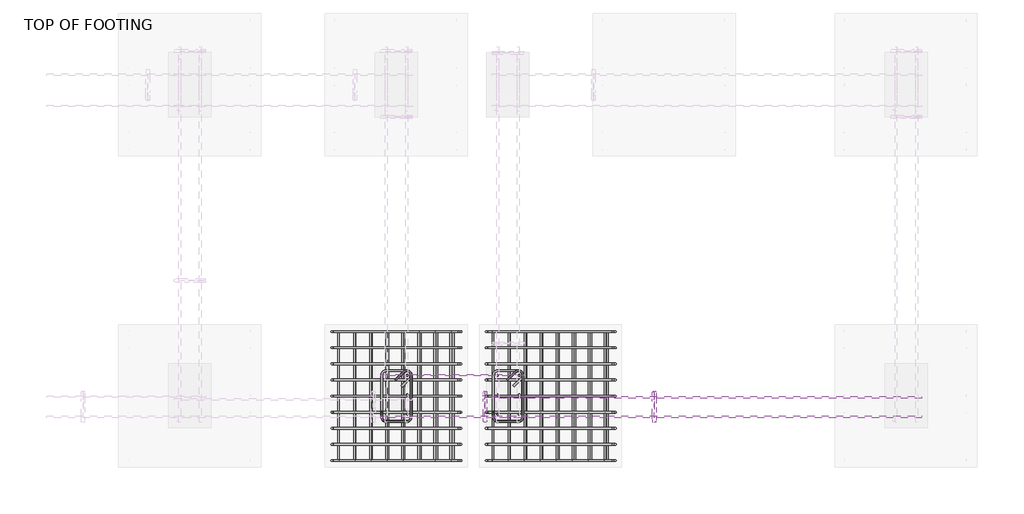
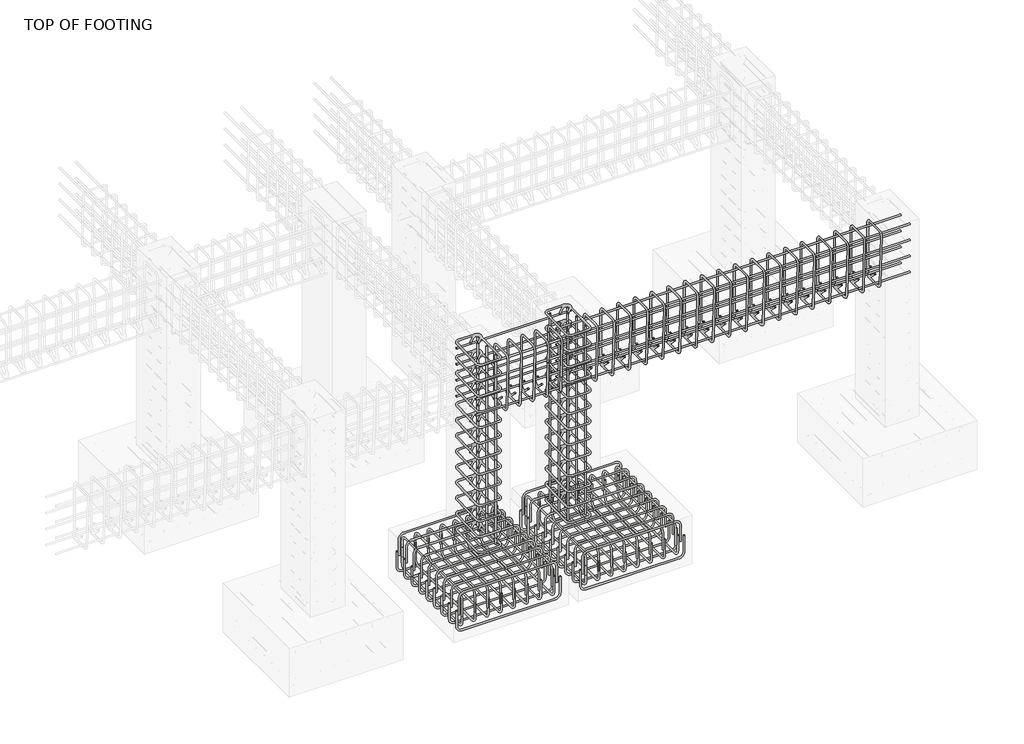
# One storey, part 3 of 19: 19 reinforcing bars.
"""IFC4 building model written with IfcOpenShell, lengths in millimetres."""

from ifc_helpers import new_model, si_unit, point, frame, origin, place, context, project, spatial, polyline, circle_curve, trimmed, segment, composite_curve, source, transform, mapped, element, save
from ifc_brep_helpers import swept_disk

model = new_model("IFC4")

# Units and contexts
model_context = context("Model", 3, world=origin())
ifc_project = project(units=[si_unit("LENGTHUNIT", "METRE", prefix="MILLI")], contexts=[model_context])

# Site, building, storey
site = spatial("IfcSite", under=ifc_project)
building = spatial("IfcBuilding", under=site)
storey = spatial("IfcBuildingStorey", under=building, Name="TOP OF FOOTING", Elevation=-1828.8)

# Reinforcing bars
placement = place(None, origin())
reinforcing_bar_shape = source(origin(), model_context, "Body", "SolidModel", [
    swept_disk(composite_curve([segment(polyline([(-418.7814918, -464.2751006, -2026.8103972), (-418.7814918, -464.2751006, -2174.1103972)]), True, "CONTINUOUS"), segment(trimmed(circle_curve(frame((-465.1314918, -464.2751006, -2174.1103972), z_axis=(0.0, 1.0, 0.0), x_axis=(46.349999999999966, 0.0, 0.0)), 46.35), [point((-418.7814918, -464.2751006, -2174.1103972))], [point((-465.1314918, -464.2751006, -2220.4603972))], True, "CARTESIAN"), True, "CONTINUOUS"), segment(polyline([(-465.1314918, -464.2751006, -2220.4603972), (-1279.7314918, -464.2751006, -2220.4603972)]), True, "CONTINUOUS"), segment(trimmed(circle_curve(frame((-1279.7314918, -464.2751006, -2174.1103972), z_axis=(0.0, 1.0, 0.0), x_axis=(0.0, 0.0, -46.34999999999991)), 46.35), [point((-1279.7314918, -464.2751006, -2220.4603972))], [point((-1326.0814918, -464.2751006, -2174.1103972))], True, "CARTESIAN"), True, "CONTINUOUS"), segment(polyline([(-1326.0814918, -464.2751006, -2174.1103972), (-1326.0814918, -464.2751006, -2026.8103972)]), True, "CONTINUOUS")], self_intersect=False), 6.35),
])
element("IfcReinforcingBar", 1, at=placement, inside=storey, context=model_context, shape_type="MappedRepresentation", body=[
    mapped(reinforcing_bar_shape, transform((0.0, 0.0, 0.0), x_axis=(1.0, 0.0, 0.0), y_axis=(0.0, 1.0, 0.0), z_axis=(0.0, 0.0, 1.0))),
    mapped(reinforcing_bar_shape, transform((0.0, -113.4125, 0.0), x_axis=(1.0, 0.0, 0.0), y_axis=(0.0, 1.0, 0.0), z_axis=(0.0, 0.0, 1.0))),
    mapped(reinforcing_bar_shape, transform((0.0, -226.825, 0.0), x_axis=(1.0, 0.0, 0.0), y_axis=(0.0, 1.0, 0.0), z_axis=(0.0, 0.0, 1.0))),
    mapped(reinforcing_bar_shape, transform((0.0, -340.2375, 0.0), x_axis=(1.0, 0.0, 0.0), y_axis=(0.0, 1.0, 0.0), z_axis=(0.0, 0.0, 1.0))),
    mapped(reinforcing_bar_shape, transform((0.0, -453.65, 0.0), x_axis=(1.0, 0.0, 0.0), y_axis=(0.0, 1.0, 0.0), z_axis=(0.0, 0.0, 1.0))),
    mapped(reinforcing_bar_shape, transform((0.0, -567.0625, 0.0), x_axis=(1.0, 0.0, 0.0), y_axis=(0.0, 1.0, 0.0), z_axis=(0.0, 0.0, 1.0))),
    mapped(reinforcing_bar_shape, transform((0.0, -680.475, 0.0), x_axis=(1.0, 0.0, 0.0), y_axis=(0.0, 1.0, 0.0), z_axis=(0.0, 0.0, 1.0))),
    mapped(reinforcing_bar_shape, transform((0.0, -793.8875, 0.0), x_axis=(1.0, 0.0, 0.0), y_axis=(0.0, 1.0, 0.0), z_axis=(0.0, 0.0, 1.0))),
    mapped(reinforcing_bar_shape, transform((0.0, -907.3, 0.0), x_axis=(1.0, 0.0, 0.0), y_axis=(0.0, 1.0, 0.0), z_axis=(0.0, 0.0, 1.0))),
])
reinforcing_bar_2_shape = source(origin(), model_context, "Body", "SolidModel", [
    swept_disk(composite_curve([segment(polyline([(-1306.5435207, -464.2751006, -2068.8), (-1306.5435207, -464.2751006, -1921.5)]), True, "CONTINUOUS"), segment(trimmed(circle_curve(frame((-1260.1935207, -464.2751006, -1921.5), z_axis=(0.0, 1.0, 0.0), x_axis=(-46.350000000000136, 0.0, 0.0)), 46.35), [point((-1306.5435207, -464.2751006, -1921.5))], [point((-1260.1935207, -464.2751006, -1875.15))], True, "CARTESIAN"), True, "CONTINUOUS"), segment(polyline([(-1260.1935207, -464.2751006, -1875.15), (-495.0610019, -464.2751006, -1875.15)]), True, "CONTINUOUS"), segment(trimmed(circle_curve(frame((-495.0610019, -464.2751006, -1921.5), z_axis=(0.0, 1.0, 0.0), x_axis=(0.0, 0.0, 46.34999999999991)), 46.35), [point((-495.0610019, -464.2751006, -1875.15))], [point((-448.7110019, -464.2751006, -1921.5))], True, "CARTESIAN"), True, "CONTINUOUS"), segment(polyline([(-448.7110019, -464.2751006, -1921.5), (-448.7110019, -464.2751006, -2068.8)]), True, "CONTINUOUS")], self_intersect=False), 6.35),
])
element("IfcReinforcingBar", 2, at=placement, inside=storey, context=model_context, shape_type="MappedRepresentation", body=[
    mapped(reinforcing_bar_2_shape, transform((0.0, 0.0, 0.0), x_axis=(1.0, 0.0, 0.0), y_axis=(0.0, 1.0, 0.0), z_axis=(0.0, 0.0, 1.0))),
    mapped(reinforcing_bar_2_shape, transform((0.0, -113.4125, 0.0), x_axis=(1.0, 0.0, 0.0), y_axis=(0.0, 1.0, 0.0), z_axis=(0.0, 0.0, 1.0))),
    mapped(reinforcing_bar_2_shape, transform((0.0, -226.825, 0.0), x_axis=(1.0, 0.0, 0.0), y_axis=(0.0, 1.0, 0.0), z_axis=(0.0, 0.0, 1.0))),
    mapped(reinforcing_bar_2_shape, transform((0.0, -340.2375, 0.0), x_axis=(1.0, 0.0, 0.0), y_axis=(0.0, 1.0, 0.0), z_axis=(0.0, 0.0, 1.0))),
    mapped(reinforcing_bar_2_shape, transform((0.0, -453.65, 0.0), x_axis=(1.0, 0.0, 0.0), y_axis=(0.0, 1.0, 0.0), z_axis=(0.0, 0.0, 1.0))),
    mapped(reinforcing_bar_2_shape, transform((0.0, -567.0625, 0.0), x_axis=(1.0, 0.0, 0.0), y_axis=(0.0, 1.0, 0.0), z_axis=(0.0, 0.0, 1.0))),
    mapped(reinforcing_bar_2_shape, transform((0.0, -680.475, 0.0), x_axis=(1.0, 0.0, 0.0), y_axis=(0.0, 1.0, 0.0), z_axis=(0.0, 0.0, 1.0))),
    mapped(reinforcing_bar_2_shape, transform((0.0, -793.8875, 0.0), x_axis=(1.0, 0.0, 0.0), y_axis=(0.0, 1.0, 0.0), z_axis=(0.0, 0.0, 1.0))),
    mapped(reinforcing_bar_2_shape, transform((0.0, -907.3, 0.0), x_axis=(1.0, 0.0, 0.0), y_axis=(0.0, 1.0, 0.0), z_axis=(0.0, 0.0, 1.0))),
])
reinforcing_bar_3_shape = source(origin(), model_context, "Body", "SolidModel", [
    swept_disk(composite_curve([segment(polyline([(-491.2862984, -464.2751006, -2090.0818702), (-491.2862984, -464.2751006, -1942.7818702)]), True, "CONTINUOUS"), segment(trimmed(circle_curve(frame((-491.2862984, -510.6251006, -1942.7818702), z_axis=(1.0, 0.0, 0.0), x_axis=(0.0, 46.35000000000002, 0.0)), 46.35), [point((-491.2862984, -464.2751006, -1942.7818702))], [point((-491.2862984, -510.6251006, -1896.4318702))], True, "CARTESIAN"), True, "CONTINUOUS"), segment(polyline([(-491.2862984, -510.6251006, -1896.4318702), (-491.2862984, -1325.2251006, -1896.4318702)]), True, "CONTINUOUS"), segment(trimmed(circle_curve(frame((-491.2862984, -1325.2251006, -1942.7818702), z_axis=(1.0, 0.0, 0.0), x_axis=(0.0, 0.0, 46.34999999999991)), 46.35), [point((-491.2862984, -1325.2251006, -1896.4318702))], [point((-491.2862984, -1371.5751006, -1942.7818702))], True, "CARTESIAN"), True, "CONTINUOUS"), segment(polyline([(-491.2862984, -1371.5751006, -1942.7818702), (-491.2862984, -1371.5751006, -2090.0818702)]), True, "CONTINUOUS")], self_intersect=False), 6.35),
])
element("IfcReinforcingBar", 3, at=placement, inside=storey, context=model_context, shape_type="MappedRepresentation", body=[
    mapped(reinforcing_bar_3_shape, transform((0.0, 0.0, 0.0), x_axis=(1.0, 0.0, 0.0), y_axis=(0.0, 1.0, 0.0), z_axis=(0.0, 0.0, 1.0))),
    mapped(reinforcing_bar_3_shape, transform((-112.5756498, 0.0, 0.0), x_axis=(1.0, 0.0, 0.0), y_axis=(0.0, 1.0, 0.0), z_axis=(0.0, 0.0, 1.0))),
    mapped(reinforcing_bar_3_shape, transform((-225.1512997, 0.0, 0.0), x_axis=(1.0, 0.0, 0.0), y_axis=(0.0, 1.0, 0.0), z_axis=(0.0, 0.0, 1.0))),
    mapped(reinforcing_bar_3_shape, transform((-337.7269495, 0.0, 0.0), x_axis=(1.0, 0.0, 0.0), y_axis=(0.0, 1.0, 0.0), z_axis=(0.0, 0.0, 1.0))),
    mapped(reinforcing_bar_3_shape, transform((-450.3025994, 0.0, 0.0), x_axis=(1.0, 0.0, 0.0), y_axis=(0.0, 1.0, 0.0), z_axis=(0.0, 0.0, 1.0))),
    mapped(reinforcing_bar_3_shape, transform((-562.8782492, 0.0, 0.0), x_axis=(1.0, 0.0, 0.0), y_axis=(0.0, 1.0, 0.0), z_axis=(0.0, 0.0, 1.0))),
    mapped(reinforcing_bar_3_shape, transform((-675.4538991, 0.0, 0.0), x_axis=(1.0, 0.0, 0.0), y_axis=(0.0, 1.0, 0.0), z_axis=(0.0, 0.0, 1.0))),
    mapped(reinforcing_bar_3_shape, transform((-788.0295489, 0.0, 0.0), x_axis=(1.0, 0.0, 0.0), y_axis=(0.0, 1.0, 0.0), z_axis=(0.0, 0.0, 1.0))),
])
reinforcing_bar_4_shape = source(origin(), model_context, "Body", "SolidModel", [
    swept_disk(composite_curve([segment(polyline([(-1279.3158473, -464.2751006, -2000.9061905), (-1279.3158473, -464.2751006, -2148.2061905)]), True, "CONTINUOUS"), segment(trimmed(circle_curve(frame((-1279.3158473, -510.6251006, -2148.2061905), z_axis=(-1.0, 0.0, 0.0), x_axis=(0.0, 46.35000000000002, 0.0)), 46.35), [point((-1279.3158473, -464.2751006, -2148.2061905))], [point((-1279.3158473, -510.6251006, -2194.5561905))], True, "CARTESIAN"), True, "CONTINUOUS"), segment(polyline([(-1279.3158473, -510.6251006, -2194.5561905), (-1279.3158473, -1325.2251006, -2194.5561905)]), True, "CONTINUOUS"), segment(trimmed(circle_curve(frame((-1279.3158473, -1325.2251006, -2148.2061905), z_axis=(-1.0, 0.0, 0.0), x_axis=(0.0, 0.0, -46.34999999999991)), 46.35), [point((-1279.3158473, -1325.2251006, -2194.5561905))], [point((-1279.3158473, -1371.5751006, -2148.2061905))], True, "CARTESIAN"), True, "CONTINUOUS"), segment(polyline([(-1279.3158473, -1371.5751006, -2148.2061905), (-1279.3158473, -1371.5751006, -2000.9061905)]), True, "CONTINUOUS")], self_intersect=False), 6.35),
])
element("IfcReinforcingBar", 4, at=placement, inside=storey, context=model_context, shape_type="MappedRepresentation", body=[
    mapped(reinforcing_bar_4_shape, transform((0.0, 0.0, 0.0), x_axis=(1.0, 0.0, 0.0), y_axis=(0.0, 1.0, 0.0), z_axis=(0.0, 0.0, 1.0))),
    mapped(reinforcing_bar_4_shape, transform((115.0727115, 0.0, 0.0), x_axis=(1.0, 0.0, 0.0), y_axis=(0.0, 1.0, 0.0), z_axis=(0.0, 0.0, 1.0))),
    mapped(reinforcing_bar_4_shape, transform((230.145423, 0.0, 0.0), x_axis=(1.0, 0.0, 0.0), y_axis=(0.0, 1.0, 0.0), z_axis=(0.0, 0.0, 1.0))),
    mapped(reinforcing_bar_4_shape, transform((345.2181344, 0.0, 0.0), x_axis=(1.0, 0.0, 0.0), y_axis=(0.0, 1.0, 0.0), z_axis=(0.0, 0.0, 1.0))),
    mapped(reinforcing_bar_4_shape, transform((460.2908459, 0.0, 0.0), x_axis=(1.0, 0.0, 0.0), y_axis=(0.0, 1.0, 0.0), z_axis=(0.0, 0.0, 1.0))),
    mapped(reinforcing_bar_4_shape, transform((575.3635574, 0.0, 0.0), x_axis=(1.0, 0.0, 0.0), y_axis=(0.0, 1.0, 0.0), z_axis=(0.0, 0.0, 1.0))),
    mapped(reinforcing_bar_4_shape, transform((690.4362689, 0.0, 0.0), x_axis=(1.0, 0.0, 0.0), y_axis=(0.0, 1.0, 0.0), z_axis=(0.0, 0.0, 1.0))),
    mapped(reinforcing_bar_4_shape, transform((805.5089804, 0.0, 0.0), x_axis=(1.0, 0.0, 0.0), y_axis=(0.0, 1.0, 0.0), z_axis=(0.0, 0.0, 1.0))),
])
reinforcing_bar_5_shape = source(origin(), model_context, "Body", "SolidModel", [
    swept_disk(composite_curve([segment(polyline([(-1504.0266954, -464.2751006, -2026.8103972), (-1504.0266954, -464.2751006, -2174.1103972)]), True, "CONTINUOUS"), segment(trimmed(circle_curve(frame((-1550.3766954, -464.2751006, -2174.1103972), z_axis=(0.0, 1.0, 0.0), x_axis=(46.34999999999991, 0.0, 0.0)), 46.35), [point((-1504.0266954, -464.2751006, -2174.1103972))], [point((-1550.3766954, -464.2751006, -2220.4603972))], True, "CARTESIAN"), True, "CONTINUOUS"), segment(polyline([(-1550.3766954, -464.2751006, -2220.4603972), (-2364.9766954, -464.2751006, -2220.4603972)]), True, "CONTINUOUS"), segment(trimmed(circle_curve(frame((-2364.9766954, -464.2751006, -2174.1103972), z_axis=(0.0, 1.0, 0.0), x_axis=(0.0, 0.0, -46.34999999999991)), 46.35), [point((-2364.9766954, -464.2751006, -2220.4603972))], [point((-2411.3266954, -464.2751006, -2174.1103972))], True, "CARTESIAN"), True, "CONTINUOUS"), segment(polyline([(-2411.3266954, -464.2751006, -2174.1103972), (-2411.3266954, -464.2751006, -2026.8103972)]), True, "CONTINUOUS")], self_intersect=False), 6.35),
])
element("IfcReinforcingBar", 5, at=placement, inside=storey, context=model_context, shape_type="MappedRepresentation", body=[
    mapped(reinforcing_bar_5_shape, transform((0.0, 0.0, 0.0), x_axis=(1.0, 0.0, 0.0), y_axis=(0.0, 1.0, 0.0), z_axis=(0.0, 0.0, 1.0))),
    mapped(reinforcing_bar_5_shape, transform((0.0, -113.4125, 0.0), x_axis=(1.0, 0.0, 0.0), y_axis=(0.0, 1.0, 0.0), z_axis=(0.0, 0.0, 1.0))),
    mapped(reinforcing_bar_5_shape, transform((0.0, -226.825, 0.0), x_axis=(1.0, 0.0, 0.0), y_axis=(0.0, 1.0, 0.0), z_axis=(0.0, 0.0, 1.0))),
    mapped(reinforcing_bar_5_shape, transform((0.0, -340.2375, 0.0), x_axis=(1.0, 0.0, 0.0), y_axis=(0.0, 1.0, 0.0), z_axis=(0.0, 0.0, 1.0))),
    mapped(reinforcing_bar_5_shape, transform((0.0, -453.65, 0.0), x_axis=(1.0, 0.0, 0.0), y_axis=(0.0, 1.0, 0.0), z_axis=(0.0, 0.0, 1.0))),
    mapped(reinforcing_bar_5_shape, transform((0.0, -567.0625, 0.0), x_axis=(1.0, 0.0, 0.0), y_axis=(0.0, 1.0, 0.0), z_axis=(0.0, 0.0, 1.0))),
    mapped(reinforcing_bar_5_shape, transform((0.0, -680.475, 0.0), x_axis=(1.0, 0.0, 0.0), y_axis=(0.0, 1.0, 0.0), z_axis=(0.0, 0.0, 1.0))),
    mapped(reinforcing_bar_5_shape, transform((0.0, -793.8875, 0.0), x_axis=(1.0, 0.0, 0.0), y_axis=(0.0, 1.0, 0.0), z_axis=(0.0, 0.0, 1.0))),
    mapped(reinforcing_bar_5_shape, transform((0.0, -907.3, 0.0), x_axis=(1.0, 0.0, 0.0), y_axis=(0.0, 1.0, 0.0), z_axis=(0.0, 0.0, 1.0))),
])
reinforcing_bar_6_shape = source(origin(), model_context, "Body", "SolidModel", [
    swept_disk(composite_curve([segment(polyline([(-2391.7887242, -464.2751006, -2068.8), (-2391.7887242, -464.2751006, -1921.5)]), True, "CONTINUOUS"), segment(trimmed(circle_curve(frame((-2345.4387242, -464.2751006, -1921.5), z_axis=(0.0, 1.0, 0.0), x_axis=(-46.350000000000364, 0.0, 0.0)), 46.35), [point((-2391.7887242, -464.2751006, -1921.5))], [point((-2345.4387242, -464.2751006, -1875.15))], True, "CARTESIAN"), True, "CONTINUOUS"), segment(polyline([(-2345.4387242, -464.2751006, -1875.15), (-1580.3062054, -464.2751006, -1875.15)]), True, "CONTINUOUS"), segment(trimmed(circle_curve(frame((-1580.3062054, -464.2751006, -1921.5), z_axis=(0.0, 1.0, 0.0), x_axis=(0.0, 0.0, 46.34999999999991)), 46.35), [point((-1580.3062054, -464.2751006, -1875.15))], [point((-1533.9562054, -464.2751006, -1921.5))], True, "CARTESIAN"), True, "CONTINUOUS"), segment(polyline([(-1533.9562054, -464.2751006, -1921.5), (-1533.9562054, -464.2751006, -2068.8)]), True, "CONTINUOUS")], self_intersect=False), 6.35),
])
element("IfcReinforcingBar", 6, at=placement, inside=storey, context=model_context, shape_type="MappedRepresentation", body=[
    mapped(reinforcing_bar_6_shape, transform((0.0, 0.0, 0.0), x_axis=(1.0, 0.0, 0.0), y_axis=(0.0, 1.0, 0.0), z_axis=(0.0, 0.0, 1.0))),
    mapped(reinforcing_bar_6_shape, transform((0.0, -113.4125, 0.0), x_axis=(1.0, 0.0, 0.0), y_axis=(0.0, 1.0, 0.0), z_axis=(0.0, 0.0, 1.0))),
    mapped(reinforcing_bar_6_shape, transform((0.0, -226.825, 0.0), x_axis=(1.0, 0.0, 0.0), y_axis=(0.0, 1.0, 0.0), z_axis=(0.0, 0.0, 1.0))),
    mapped(reinforcing_bar_6_shape, transform((0.0, -340.2375, 0.0), x_axis=(1.0, 0.0, 0.0), y_axis=(0.0, 1.0, 0.0), z_axis=(0.0, 0.0, 1.0))),
    mapped(reinforcing_bar_6_shape, transform((0.0, -453.65, 0.0), x_axis=(1.0, 0.0, 0.0), y_axis=(0.0, 1.0, 0.0), z_axis=(0.0, 0.0, 1.0))),
    mapped(reinforcing_bar_6_shape, transform((0.0, -567.0625, 0.0), x_axis=(1.0, 0.0, 0.0), y_axis=(0.0, 1.0, 0.0), z_axis=(0.0, 0.0, 1.0))),
    mapped(reinforcing_bar_6_shape, transform((0.0, -680.475, 0.0), x_axis=(1.0, 0.0, 0.0), y_axis=(0.0, 1.0, 0.0), z_axis=(0.0, 0.0, 1.0))),
    mapped(reinforcing_bar_6_shape, transform((0.0, -793.8875, 0.0), x_axis=(1.0, 0.0, 0.0), y_axis=(0.0, 1.0, 0.0), z_axis=(0.0, 0.0, 1.0))),
    mapped(reinforcing_bar_6_shape, transform((0.0, -907.3, 0.0), x_axis=(1.0, 0.0, 0.0), y_axis=(0.0, 1.0, 0.0), z_axis=(0.0, 0.0, 1.0))),
])
reinforcing_bar_7_shape = source(origin(), model_context, "Body", "SolidModel", [
    swept_disk(composite_curve([segment(polyline([(-1576.531502, -464.2751006, -2090.0818702), (-1576.531502, -464.2751006, -1942.7818702)]), True, "CONTINUOUS"), segment(trimmed(circle_curve(frame((-1576.531502, -510.6251006, -1942.7818702), z_axis=(1.0, 0.0, 0.0), x_axis=(0.0, 46.35000000000002, 0.0)), 46.35), [point((-1576.531502, -464.2751006, -1942.7818702))], [point((-1576.531502, -510.6251006, -1896.4318702))], True, "CARTESIAN"), True, "CONTINUOUS"), segment(polyline([(-1576.531502, -510.6251006, -1896.4318702), (-1576.531502, -1325.2251006, -1896.4318702)]), True, "CONTINUOUS"), segment(trimmed(circle_curve(frame((-1576.531502, -1325.2251006, -1942.7818702), z_axis=(1.0, 0.0, 0.0), x_axis=(0.0, 0.0, 46.34999999999991)), 46.35), [point((-1576.531502, -1325.2251006, -1896.4318702))], [point((-1576.531502, -1371.5751006, -1942.7818702))], True, "CARTESIAN"), True, "CONTINUOUS"), segment(polyline([(-1576.531502, -1371.5751006, -1942.7818702), (-1576.531502, -1371.5751006, -2090.0818702)]), True, "CONTINUOUS")], self_intersect=False), 6.35),
])
element("IfcReinforcingBar", 7, at=placement, inside=storey, context=model_context, shape_type="MappedRepresentation", body=[
    mapped(reinforcing_bar_7_shape, transform((0.0, 0.0, 0.0), x_axis=(1.0, 0.0, 0.0), y_axis=(0.0, 1.0, 0.0), z_axis=(0.0, 0.0, 1.0))),
    mapped(reinforcing_bar_7_shape, transform((-112.5756498, 0.0, 0.0), x_axis=(1.0, 0.0, 0.0), y_axis=(0.0, 1.0, 0.0), z_axis=(0.0, 0.0, 1.0))),
    mapped(reinforcing_bar_7_shape, transform((-225.1512997, 0.0, 0.0), x_axis=(1.0, 0.0, 0.0), y_axis=(0.0, 1.0, 0.0), z_axis=(0.0, 0.0, 1.0))),
    mapped(reinforcing_bar_7_shape, transform((-337.7269495, 0.0, 0.0), x_axis=(1.0, 0.0, 0.0), y_axis=(0.0, 1.0, 0.0), z_axis=(0.0, 0.0, 1.0))),
    mapped(reinforcing_bar_7_shape, transform((-450.3025994, 0.0, 0.0), x_axis=(1.0, 0.0, 0.0), y_axis=(0.0, 1.0, 0.0), z_axis=(0.0, 0.0, 1.0))),
    mapped(reinforcing_bar_7_shape, transform((-562.8782492, 0.0, 0.0), x_axis=(1.0, 0.0, 0.0), y_axis=(0.0, 1.0, 0.0), z_axis=(0.0, 0.0, 1.0))),
    mapped(reinforcing_bar_7_shape, transform((-675.4538991, 0.0, 0.0), x_axis=(1.0, 0.0, 0.0), y_axis=(0.0, 1.0, 0.0), z_axis=(0.0, 0.0, 1.0))),
    mapped(reinforcing_bar_7_shape, transform((-788.0295489, 0.0, 0.0), x_axis=(1.0, 0.0, 0.0), y_axis=(0.0, 1.0, 0.0), z_axis=(0.0, 0.0, 1.0))),
])
reinforcing_bar_8_shape = source(origin(), model_context, "Body", "SolidModel", [
    swept_disk(composite_curve([segment(polyline([(-2364.5610509, -464.2751006, -2000.9061905), (-2364.5610509, -464.2751006, -2148.2061905)]), True, "CONTINUOUS"), segment(trimmed(circle_curve(frame((-2364.5610509, -510.6251006, -2148.2061905), z_axis=(-1.0, 0.0, 0.0), x_axis=(0.0, 46.35000000000002, 0.0)), 46.35), [point((-2364.5610509, -464.2751006, -2148.2061905))], [point((-2364.5610509, -510.6251006, -2194.5561905))], True, "CARTESIAN"), True, "CONTINUOUS"), segment(polyline([(-2364.5610509, -510.6251006, -2194.5561905), (-2364.5610509, -1325.2251006, -2194.5561905)]), True, "CONTINUOUS"), segment(trimmed(circle_curve(frame((-2364.5610509, -1325.2251006, -2148.2061905), z_axis=(-1.0, 0.0, 0.0), x_axis=(0.0, 0.0, -46.34999999999991)), 46.35), [point((-2364.5610509, -1325.2251006, -2194.5561905))], [point((-2364.5610509, -1371.5751006, -2148.2061905))], True, "CARTESIAN"), True, "CONTINUOUS"), segment(polyline([(-2364.5610509, -1371.5751006, -2148.2061905), (-2364.5610509, -1371.5751006, -2000.9061905)]), True, "CONTINUOUS")], self_intersect=False), 6.35),
])
element("IfcReinforcingBar", 8, at=placement, inside=storey, context=model_context, shape_type="MappedRepresentation", body=[
    mapped(reinforcing_bar_8_shape, transform((0.0, 0.0, 0.0), x_axis=(1.0, 0.0, 0.0), y_axis=(0.0, 1.0, 0.0), z_axis=(0.0, 0.0, 1.0))),
    mapped(reinforcing_bar_8_shape, transform((115.0727115, 0.0, 0.0), x_axis=(1.0, 0.0, 0.0), y_axis=(0.0, 1.0, 0.0), z_axis=(0.0, 0.0, 1.0))),
    mapped(reinforcing_bar_8_shape, transform((230.145423, 0.0, 0.0), x_axis=(1.0, 0.0, 0.0), y_axis=(0.0, 1.0, 0.0), z_axis=(0.0, 0.0, 1.0))),
    mapped(reinforcing_bar_8_shape, transform((345.2181344, 0.0, 0.0), x_axis=(1.0, 0.0, 0.0), y_axis=(0.0, 1.0, 0.0), z_axis=(0.0, 0.0, 1.0))),
    mapped(reinforcing_bar_8_shape, transform((460.2908459, 0.0, 0.0), x_axis=(1.0, 0.0, 0.0), y_axis=(0.0, 1.0, 0.0), z_axis=(0.0, 0.0, 1.0))),
    mapped(reinforcing_bar_8_shape, transform((575.3635574, 0.0, 0.0), x_axis=(1.0, 0.0, 0.0), y_axis=(0.0, 1.0, 0.0), z_axis=(0.0, 0.0, 1.0))),
    mapped(reinforcing_bar_8_shape, transform((690.4362689, 0.0, 0.0), x_axis=(1.0, 0.0, 0.0), y_axis=(0.0, 1.0, 0.0), z_axis=(0.0, 0.0, 1.0))),
    mapped(reinforcing_bar_8_shape, transform((805.5089804, 0.0, 0.0), x_axis=(1.0, 0.0, 0.0), y_axis=(0.0, 1.0, 0.0), z_axis=(0.0, 0.0, 1.0))),
])
reinforcing_bar_9_shape = source(origin(), model_context, "Body", "SolidModel", [
    swept_disk(composite_curve([segment(polyline([(-1963.2880559, -804.200866, -46.35), (-1907.544493, -748.457303, -46.35)]), True, "CONTINUOUS"), segment(trimmed(circle_curve(frame((-1885.3766954, -770.6251006, -46.35), z_axis=(0.0, 0.0, -1.0), x_axis=(-22.167797600000085, 22.16779759999997, 0.0)), 31.35), [point((-1907.544493, -748.457303, -46.35))], [point((-1854.0266954, -770.6251006, -46.35))], True, "CARTESIAN"), True, "CONTINUOUS"), segment(polyline([(-1854.0266954, -770.6251006, -46.35), (-1854.0266954, -1065.2251006, -46.35)]), True, "CONTINUOUS"), segment(trimmed(circle_curve(frame((-1885.3766954, -1065.2251006, -46.35), z_axis=(0.0, 0.0, -1.0), x_axis=(31.34999999999991, 0.0, 0.0)), 31.35), [point((-1854.0266954, -1065.2251006, -46.35))], [point((-1885.3766954, -1096.5751006, -46.35))], True, "CARTESIAN"), True, "CONTINUOUS"), segment(polyline([(-1885.3766954, -1096.5751006, -46.35), (-2029.9766954, -1096.5751006, -46.35)]), True, "CONTINUOUS"), segment(trimmed(circle_curve(frame((-2029.9766954, -1065.2448857, -45.2363875), z_axis=(0.0, 0.035521928334481916, -0.9993688971583016), x_axis=(0.0, -31.3302149000001, -1.1136125000000021)), 31.35), [point((-2029.9766954, -1096.5751006, -46.35))], [point((-2061.3266954, -1065.2448857, -45.2363875))], True, "CARTESIAN"), True, "CONTINUOUS"), segment(polyline([(-2061.3266954, -1065.2448857, -45.2363875), (-2061.3266954, -770.6053156, -34.7636125)]), True, "CONTINUOUS"), segment(trimmed(circle_curve(frame((-2029.9766954, -770.6053156, -34.7636125), z_axis=(0.0, 0.035521928334481916, -0.9993688971583016), x_axis=(-31.350000000000136, 0.0, 0.0)), 31.35), [point((-2061.3266954, -770.6053156, -34.7636125))], [point((-2029.9766954, -739.2751006, -33.65))], True, "CARTESIAN"), True, "CONTINUOUS"), segment(polyline([(-2029.9766954, -739.2751006, -33.65), (-1885.3766954, -739.2751006, -33.65)]), True, "CONTINUOUS"), segment(trimmed(circle_curve(frame((-1885.3766954, -770.6251006, -33.65), z_axis=(0.0, 0.0, -1.0), x_axis=(0.0, 31.350000000000023, 0.0)), 31.35), [point((-1885.3766954, -739.2751006, -33.65))], [point((-1863.2088978, -792.7928982, -33.65))], True, "CARTESIAN"), True, "CONTINUOUS"), segment(polyline([(-1863.2088978, -792.7928982, -33.65), (-1918.9524607, -848.5364612, -33.65)]), True, "CONTINUOUS")], self_intersect=False), 6.35),
])
element("IfcReinforcingBar", 9, at=placement, inside=storey, context=model_context, shape_type="MappedRepresentation", body=[
    mapped(reinforcing_bar_9_shape, transform((0.0, 0.0, 0.0), x_axis=(1.0, 0.0, 0.0), y_axis=(0.0, 1.0, 0.0), z_axis=(0.0, 0.0, 1.0))),
    mapped(reinforcing_bar_9_shape, transform((0.0, 0.0, -144.675), x_axis=(1.0, 0.0, 0.0), y_axis=(0.0, 1.0, 0.0), z_axis=(0.0, 0.0, 1.0))),
    mapped(reinforcing_bar_9_shape, transform((0.0, 0.0, -289.35), x_axis=(1.0, 0.0, 0.0), y_axis=(0.0, 1.0, 0.0), z_axis=(0.0, 0.0, 1.0))),
    mapped(reinforcing_bar_9_shape, transform((0.0, 0.0, -434.025), x_axis=(1.0, 0.0, 0.0), y_axis=(0.0, 1.0, 0.0), z_axis=(0.0, 0.0, 1.0))),
    mapped(reinforcing_bar_9_shape, transform((0.0, 0.0, -578.7), x_axis=(1.0, 0.0, 0.0), y_axis=(0.0, 1.0, 0.0), z_axis=(0.0, 0.0, 1.0))),
    mapped(reinforcing_bar_9_shape, transform((0.0, 0.0, -723.375), x_axis=(1.0, 0.0, 0.0), y_axis=(0.0, 1.0, 0.0), z_axis=(0.0, 0.0, 1.0))),
    mapped(reinforcing_bar_9_shape, transform((0.0, 0.0, -868.05), x_axis=(1.0, 0.0, 0.0), y_axis=(0.0, 1.0, 0.0), z_axis=(0.0, 0.0, 1.0))),
    mapped(reinforcing_bar_9_shape, transform((0.0, 0.0, -1012.725), x_axis=(1.0, 0.0, 0.0), y_axis=(0.0, 1.0, 0.0), z_axis=(0.0, 0.0, 1.0))),
    mapped(reinforcing_bar_9_shape, transform((0.0, 0.0, -1157.4), x_axis=(1.0, 0.0, 0.0), y_axis=(0.0, 1.0, 0.0), z_axis=(0.0, 0.0, 1.0))),
    mapped(reinforcing_bar_9_shape, transform((0.0, 0.0, -1302.075), x_axis=(1.0, 0.0, 0.0), y_axis=(0.0, 1.0, 0.0), z_axis=(0.0, 0.0, 1.0))),
    mapped(reinforcing_bar_9_shape, transform((0.0, 0.0, -1446.75), x_axis=(1.0, 0.0, 0.0), y_axis=(0.0, 1.0, 0.0), z_axis=(0.0, 0.0, 1.0))),
    mapped(reinforcing_bar_9_shape, transform((0.0, 0.0, -1591.425), x_axis=(1.0, 0.0, 0.0), y_axis=(0.0, 1.0, 0.0), z_axis=(0.0, 0.0, 1.0))),
    mapped(reinforcing_bar_9_shape, transform((0.0, 0.0, -1736.1), x_axis=(1.0, 0.0, 0.0), y_axis=(0.0, 1.0, 0.0), z_axis=(0.0, 0.0, 1.0))),
])
reinforcing_bar_10_shape = source(origin(), model_context, "Body", "SolidModel", [
    swept_disk(composite_curve([segment(polyline([(-1880.3766954, -772.4299352, -40.0), (-1880.3766954, -772.4299352, -1788.8)]), True, "CONTINUOUS")], self_intersect=False), 6.35),
])
element("IfcReinforcingBar", 10, at=placement, inside=storey, context=model_context, shape_type="MappedRepresentation", body=[
    mapped(reinforcing_bar_10_shape, transform((0.0, 0.0, 0.0), x_axis=(1.0, 0.0, 0.0), y_axis=(0.0, 1.0, 0.0), z_axis=(0.0, 0.0, 1.0))),
    mapped(reinforcing_bar_10_shape, transform((0.0, -136.8171118, 0.0), x_axis=(1.0, 0.0, 0.0), y_axis=(0.0, 1.0, 0.0), z_axis=(0.0, 0.0, 1.0))),
    mapped(reinforcing_bar_10_shape, transform((0.0, -273.6342236, 0.0), x_axis=(1.0, 0.0, 0.0), y_axis=(0.0, 1.0, 0.0), z_axis=(0.0, 0.0, 1.0))),
])
reinforcing_bar_11_shape = source(origin(), model_context, "Body", "SolidModel", [
    swept_disk(composite_curve([segment(polyline([(-1178.0428523, -804.200866, -46.35), (-1122.2992894, -748.457303, -46.35)]), True, "CONTINUOUS"), segment(trimmed(circle_curve(frame((-1100.1314918, -770.6251006, -46.35), z_axis=(0.0, 0.0, -1.0), x_axis=(-22.167797599999858, 22.16779759999997, 0.0)), 31.35), [point((-1122.2992894, -748.457303, -46.35))], [point((-1068.7814918, -770.6251006, -46.35))], True, "CARTESIAN"), True, "CONTINUOUS"), segment(polyline([(-1068.7814918, -770.6251006, -46.35), (-1068.7814918, -1065.2251006, -46.35)]), True, "CONTINUOUS"), segment(trimmed(circle_curve(frame((-1100.1314918, -1065.2251006, -46.35), z_axis=(0.0, 0.0, -1.0), x_axis=(31.350000000000136, 0.0, 0.0)), 31.35), [point((-1068.7814918, -1065.2251006, -46.35))], [point((-1100.1314918, -1096.5751006, -46.35))], True, "CARTESIAN"), True, "CONTINUOUS"), segment(polyline([(-1100.1314918, -1096.5751006, -46.35), (-1244.7314918, -1096.5751006, -46.35)]), True, "CONTINUOUS"), segment(trimmed(circle_curve(frame((-1244.7314918, -1065.2448857, -45.2363875), z_axis=(0.0, 0.035521928334481916, -0.9993688971583016), x_axis=(0.0, -31.3302149000001, -1.1136125000000021)), 31.35), [point((-1244.7314918, -1096.5751006, -46.35))], [point((-1276.0814918, -1065.2448857, -45.2363875))], True, "CARTESIAN"), True, "CONTINUOUS"), segment(polyline([(-1276.0814918, -1065.2448857, -45.2363875), (-1276.0814918, -770.6053156, -34.7636125)]), True, "CONTINUOUS"), segment(trimmed(circle_curve(frame((-1244.7314918, -770.6053156, -34.7636125), z_axis=(0.0, 0.035521928334481916, -0.9993688971583016), x_axis=(-31.350000000000136, 0.0, 0.0)), 31.35), [point((-1276.0814918, -770.6053156, -34.7636125))], [point((-1244.7314918, -739.2751006, -33.65))], True, "CARTESIAN"), True, "CONTINUOUS"), segment(polyline([(-1244.7314918, -739.2751006, -33.65), (-1100.1314918, -739.2751006, -33.65)]), True, "CONTINUOUS"), segment(trimmed(circle_curve(frame((-1100.1314918, -770.6251006, -33.65), z_axis=(0.0, 0.0, -1.0), x_axis=(0.0, 31.350000000000023, 0.0)), 31.35), [point((-1100.1314918, -739.2751006, -33.65))], [point((-1077.9636942, -792.7928982, -33.65))], True, "CARTESIAN"), True, "CONTINUOUS"), segment(polyline([(-1077.9636942, -792.7928982, -33.65), (-1133.7072572, -848.5364612, -33.65)]), True, "CONTINUOUS")], self_intersect=False), 6.35),
])
element("IfcReinforcingBar", 11, at=placement, inside=storey, context=model_context, shape_type="MappedRepresentation", body=[
    mapped(reinforcing_bar_11_shape, transform((0.0, 0.0, 0.0), x_axis=(1.0, 0.0, 0.0), y_axis=(0.0, 1.0, 0.0), z_axis=(0.0, 0.0, 1.0))),
    mapped(reinforcing_bar_11_shape, transform((0.0, 0.0, -144.675), x_axis=(1.0, 0.0, 0.0), y_axis=(0.0, 1.0, 0.0), z_axis=(0.0, 0.0, 1.0))),
    mapped(reinforcing_bar_11_shape, transform((0.0, 0.0, -289.35), x_axis=(1.0, 0.0, 0.0), y_axis=(0.0, 1.0, 0.0), z_axis=(0.0, 0.0, 1.0))),
    mapped(reinforcing_bar_11_shape, transform((0.0, 0.0, -434.025), x_axis=(1.0, 0.0, 0.0), y_axis=(0.0, 1.0, 0.0), z_axis=(0.0, 0.0, 1.0))),
    mapped(reinforcing_bar_11_shape, transform((0.0, 0.0, -578.7), x_axis=(1.0, 0.0, 0.0), y_axis=(0.0, 1.0, 0.0), z_axis=(0.0, 0.0, 1.0))),
    mapped(reinforcing_bar_11_shape, transform((0.0, 0.0, -723.375), x_axis=(1.0, 0.0, 0.0), y_axis=(0.0, 1.0, 0.0), z_axis=(0.0, 0.0, 1.0))),
    mapped(reinforcing_bar_11_shape, transform((0.0, 0.0, -868.05), x_axis=(1.0, 0.0, 0.0), y_axis=(0.0, 1.0, 0.0), z_axis=(0.0, 0.0, 1.0))),
    mapped(reinforcing_bar_11_shape, transform((0.0, 0.0, -1012.725), x_axis=(1.0, 0.0, 0.0), y_axis=(0.0, 1.0, 0.0), z_axis=(0.0, 0.0, 1.0))),
    mapped(reinforcing_bar_11_shape, transform((0.0, 0.0, -1157.4), x_axis=(1.0, 0.0, 0.0), y_axis=(0.0, 1.0, 0.0), z_axis=(0.0, 0.0, 1.0))),
    mapped(reinforcing_bar_11_shape, transform((0.0, 0.0, -1302.075), x_axis=(1.0, 0.0, 0.0), y_axis=(0.0, 1.0, 0.0), z_axis=(0.0, 0.0, 1.0))),
    mapped(reinforcing_bar_11_shape, transform((0.0, 0.0, -1446.75), x_axis=(1.0, 0.0, 0.0), y_axis=(0.0, 1.0, 0.0), z_axis=(0.0, 0.0, 1.0))),
    mapped(reinforcing_bar_11_shape, transform((0.0, 0.0, -1591.425), x_axis=(1.0, 0.0, 0.0), y_axis=(0.0, 1.0, 0.0), z_axis=(0.0, 0.0, 1.0))),
    mapped(reinforcing_bar_11_shape, transform((0.0, 0.0, -1736.1), x_axis=(1.0, 0.0, 0.0), y_axis=(0.0, 1.0, 0.0), z_axis=(0.0, 0.0, 1.0))),
])
reinforcing_bar_12_shape = source(origin(), model_context, "Body", "SolidModel", [
    swept_disk(composite_curve([segment(polyline([(-1095.1314918, -772.4299352, -40.0), (-1095.1314918, -772.4299352, -1788.8)]), True, "CONTINUOUS")], self_intersect=False), 6.35),
])
element("IfcReinforcingBar", 12, at=placement, inside=storey, context=model_context, shape_type="MappedRepresentation", body=[
    mapped(reinforcing_bar_12_shape, transform((0.0, 0.0, 0.0), x_axis=(1.0, 0.0, 0.0), y_axis=(0.0, 1.0, 0.0), z_axis=(0.0, 0.0, 1.0))),
    mapped(reinforcing_bar_12_shape, transform((0.0, -136.8171118, 0.0), x_axis=(1.0, 0.0, 0.0), y_axis=(0.0, 1.0, 0.0), z_axis=(0.0, 0.0, 1.0))),
    mapped(reinforcing_bar_12_shape, transform((0.0, -273.6342236, 0.0), x_axis=(1.0, 0.0, 0.0), y_axis=(0.0, 1.0, 0.0), z_axis=(0.0, 0.0, 1.0))),
])
reinforcing_bar_13_shape = source(origin(), model_context, "Body", "SolidModel", [
    swept_disk(composite_curve([segment(polyline([(-1247.2314918, -772.4299352, -40.0), (-1247.2314918, -772.4299352, -1788.8)]), True, "CONTINUOUS")], self_intersect=False), 6.35),
])
element("IfcReinforcingBar", 13, at=placement, inside=storey, context=model_context, shape_type="MappedRepresentation", body=[
    mapped(reinforcing_bar_13_shape, transform((0.0, 0.0, 0.0), x_axis=(1.0, 0.0, 0.0), y_axis=(0.0, 1.0, 0.0), z_axis=(0.0, 0.0, 1.0))),
    mapped(reinforcing_bar_13_shape, transform((0.0, -136.8171118, 0.0), x_axis=(1.0, 0.0, 0.0), y_axis=(0.0, 1.0, 0.0), z_axis=(0.0, 0.0, 1.0))),
    mapped(reinforcing_bar_13_shape, transform((0.0, -273.6342236, 0.0), x_axis=(1.0, 0.0, 0.0), y_axis=(0.0, 1.0, 0.0), z_axis=(0.0, 0.0, 1.0))),
])
reinforcing_bar_14_shape = source(origin(), model_context, "Body", "SolidModel", [
    swept_disk(composite_curve([segment(polyline([(-1801.3266948, -998.5364612, -488.7242346), (-1801.3266948, -942.7928982, -544.4677976)]), True, "CONTINUOUS"), segment(trimmed(circle_curve(frame((-1801.3266948, -920.6251006, -522.3), z_axis=(1.0, 0.0, 0.0), x_axis=(0.0, -22.16779759999997, -22.167797600000085)), 31.35), [point((-1801.3266948, -942.7928982, -544.4677976))], [point((-1801.3266948, -889.2751006, -522.3))], True, "CARTESIAN"), True, "CONTINUOUS"), segment(polyline([(-1801.3266948, -889.2751006, -522.3), (-1801.3266948, -889.2751006, -77.7)]), True, "CONTINUOUS"), segment(trimmed(circle_curve(frame((-1801.3266948, -920.6251006, -77.7), z_axis=(1.0, 0.0, 0.0), x_axis=(0.0, 31.350000000000023, 0.0)), 31.35), [point((-1801.3266948, -889.2751006, -77.7))], [point((-1801.3266948, -920.6251006, -46.35))], True, "CARTESIAN"), True, "CONTINUOUS"), segment(polyline([(-1801.3266948, -920.6251006, -46.35), (-1801.3266948, -1065.2251006, -46.35)]), True, "CONTINUOUS"), segment(trimmed(circle_curve(frame((-1802.1112804, -1065.2251006, -77.6901807), z_axis=(0.9996867842138424, 0.0, -0.025026655153786322), x_axis=(0.7845855999999003, 0.0, 31.340180699999998)), 31.35), [point((-1801.3266948, -1065.2251006, -46.35))], [point((-1802.1112804, -1096.5751006, -77.6901807))], True, "CARTESIAN"), True, "CONTINUOUS"), segment(polyline([(-1802.1112804, -1096.5751006, -77.6901807), (-1813.2421091, -1096.5751006, -522.3098193)]), True, "CONTINUOUS"), segment(trimmed(circle_curve(frame((-1813.2421091, -1065.2251006, -522.3098193), z_axis=(0.9996867842138424, 0.0, -0.025026655153786322), x_axis=(0.0, -31.350000000000136, 0.0)), 31.35), [point((-1813.2421091, -1096.5751006, -522.3098193))], [point((-1814.0266948, -1065.2251006, -553.65))], True, "CARTESIAN"), True, "CONTINUOUS"), segment(polyline([(-1814.0266948, -1065.2251006, -553.65), (-1814.0266948, -920.6251006, -553.65)]), True, "CONTINUOUS"), segment(trimmed(circle_curve(frame((-1814.0266948, -920.6251006, -522.3), z_axis=(1.0, 0.0, 0.0), x_axis=(0.0, 0.0, -31.350000000000023)), 31.35), [point((-1814.0266948, -920.6251006, -553.65))], [point((-1814.0266948, -898.457303, -500.1322024))], True, "CARTESIAN"), True, "CONTINUOUS"), segment(polyline([(-1814.0266948, -898.457303, -500.1322024), (-1814.0266948, -954.200866, -444.3886395)]), True, "CONTINUOUS")], self_intersect=False), 6.35),
])
element("IfcReinforcingBar", 14, at=placement, inside=storey, context=model_context, shape_type="MappedRepresentation", body=[
    mapped(reinforcing_bar_14_shape, transform((0.0, 0.0, 0.0), x_axis=(1.0, 0.0, 0.0), y_axis=(0.0, 1.0, 0.0), z_axis=(0.0, 0.0, 1.0))),
    mapped(reinforcing_bar_14_shape, transform((118.1363007, 0.0, 0.0), x_axis=(1.0, 0.0, 0.0), y_axis=(0.0, 1.0, 0.0), z_axis=(0.0, 0.0, 1.0))),
    mapped(reinforcing_bar_14_shape, transform((236.2726015, 0.0, 0.0), x_axis=(1.0, 0.0, 0.0), y_axis=(0.0, 1.0, 0.0), z_axis=(0.0, 0.0, 1.0))),
    mapped(reinforcing_bar_14_shape, transform((354.4089022, 0.0, 0.0), x_axis=(1.0, 0.0, 0.0), y_axis=(0.0, 1.0, 0.0), z_axis=(0.0, 0.0, 1.0))),
    mapped(reinforcing_bar_14_shape, transform((472.545203, 0.0, 0.0), x_axis=(1.0, 0.0, 0.0), y_axis=(0.0, 1.0, 0.0), z_axis=(0.0, 0.0, 1.0))),
])
reinforcing_bar_15_shape = source(origin(), model_context, "Body", "SolidModel", [
    swept_disk(composite_curve([segment(polyline([(-2067.6766954, -1065.2251006, -77.1929231), (-1062.4314918, -1065.2251006, -77.1929231)]), True, "CONTINUOUS")], self_intersect=False), 6.35),
])
element("IfcReinforcingBar", 15, at=placement, inside=storey, context=model_context, shape_type="MappedRepresentation", body=[
    mapped(reinforcing_bar_15_shape, transform((0.0, 0.0, 0.0), x_axis=(1.0, 0.0, 0.0), y_axis=(0.0, 1.0, 0.0), z_axis=(0.0, 0.0, 1.0))),
    mapped(reinforcing_bar_15_shape, transform((0.0, 0.0, -147.8786553), x_axis=(1.0, 0.0, 0.0), y_axis=(0.0, 1.0, 0.0), z_axis=(0.0, 0.0, 1.0))),
    mapped(reinforcing_bar_15_shape, transform((0.0, 0.0, -295.7573105), x_axis=(1.0, 0.0, 0.0), y_axis=(0.0, 1.0, 0.0), z_axis=(0.0, 0.0, 1.0))),
    mapped(reinforcing_bar_15_shape, transform((0.0, 0.0, -443.6359658), x_axis=(1.0, 0.0, 0.0), y_axis=(0.0, 1.0, 0.0), z_axis=(0.0, 0.0, 1.0))),
])
reinforcing_bar_16_shape = source(origin(), model_context, "Body", "SolidModel", [
    swept_disk(composite_curve([segment(polyline([(-2067.6766954, -770.6251006, -77.1929231), (-1062.4314918, -770.6251006, -77.1929231)]), True, "CONTINUOUS")], self_intersect=False), 6.35),
])
element("IfcReinforcingBar", 16, at=placement, inside=storey, context=model_context, shape_type="MappedRepresentation", body=[
    mapped(reinforcing_bar_16_shape, transform((0.0, 0.0, 0.0), x_axis=(1.0, 0.0, 0.0), y_axis=(0.0, 1.0, 0.0), z_axis=(0.0, 0.0, 1.0))),
    mapped(reinforcing_bar_16_shape, transform((0.0, 0.0, -147.8786553), x_axis=(1.0, 0.0, 0.0), y_axis=(0.0, 1.0, 0.0), z_axis=(0.0, 0.0, 1.0))),
    mapped(reinforcing_bar_16_shape, transform((0.0, 0.0, -295.7573105), x_axis=(1.0, 0.0, 0.0), y_axis=(0.0, 1.0, 0.0), z_axis=(0.0, 0.0, 1.0))),
    mapped(reinforcing_bar_16_shape, transform((0.0, 0.0, -443.6359658), x_axis=(1.0, 0.0, 0.0), y_axis=(0.0, 1.0, 0.0), z_axis=(0.0, 0.0, 1.0))),
])
reinforcing_bar_17_shape = source(origin(), model_context, "Body", "SolidModel", [
    swept_disk(composite_curve([segment(polyline([(-1016.0814912, -998.5364612, -488.7242346), (-1016.0814912, -942.7928982, -544.4677976)]), True, "CONTINUOUS"), segment(trimmed(circle_curve(frame((-1016.0814912, -920.6251006, -522.3), z_axis=(1.0, 0.0, 0.0), x_axis=(0.0, -22.16779759999997, -22.167797600000085)), 31.35), [point((-1016.0814912, -942.7928982, -544.4677976))], [point((-1016.0814912, -889.2751006, -522.3))], True, "CARTESIAN"), True, "CONTINUOUS"), segment(polyline([(-1016.0814912, -889.2751006, -522.3), (-1016.0814912, -889.2751006, -77.7)]), True, "CONTINUOUS"), segment(trimmed(circle_curve(frame((-1016.0814912, -920.6251006, -77.7), z_axis=(1.0, 0.0, 0.0), x_axis=(0.0, 31.350000000000023, 0.0)), 31.35), [point((-1016.0814912, -889.2751006, -77.7))], [point((-1016.0814912, -920.6251006, -46.35))], True, "CARTESIAN"), True, "CONTINUOUS"), segment(polyline([(-1016.0814912, -920.6251006, -46.35), (-1016.0814912, -1065.2251006, -46.35)]), True, "CONTINUOUS"), segment(trimmed(circle_curve(frame((-1016.8660768, -1065.2251006, -77.6901807), z_axis=(0.9996867842138424, 0.0, -0.025026655153786322), x_axis=(0.784585600000014, 0.0, 31.340180699999998)), 31.35), [point((-1016.0814912, -1065.2251006, -46.35))], [point((-1016.8660768, -1096.5751006, -77.6901807))], True, "CARTESIAN"), True, "CONTINUOUS"), segment(polyline([(-1016.8660768, -1096.5751006, -77.6901807), (-1027.9969056, -1096.5751006, -522.3098193)]), True, "CONTINUOUS"), segment(trimmed(circle_curve(frame((-1027.9969056, -1065.2251006, -522.3098193), z_axis=(0.9996867842138424, 0.0, -0.025026655153786322), x_axis=(0.0, -31.350000000000136, 0.0)), 31.35), [point((-1027.9969056, -1096.5751006, -522.3098193))], [point((-1028.7814912, -1065.2251006, -553.65))], True, "CARTESIAN"), True, "CONTINUOUS"), segment(polyline([(-1028.7814912, -1065.2251006, -553.65), (-1028.7814912, -920.6251006, -553.65)]), True, "CONTINUOUS"), segment(trimmed(circle_curve(frame((-1028.7814912, -920.6251006, -522.3), z_axis=(1.0, 0.0, 0.0), x_axis=(0.0, 0.0, -31.350000000000023)), 31.35), [point((-1028.7814912, -920.6251006, -553.65))], [point((-1028.7814912, -898.457303, -500.1322024))], True, "CARTESIAN"), True, "CONTINUOUS"), segment(polyline([(-1028.7814912, -898.457303, -500.1322024), (-1028.7814912, -954.200866, -444.3886395)]), True, "CONTINUOUS")], self_intersect=False), 6.35),
])
element("IfcReinforcingBar", 17, at=placement, inside=storey, context=model_context, shape_type="MappedRepresentation", body=[
    mapped(reinforcing_bar_17_shape, transform((0.0, 0.0, 0.0), x_axis=(1.0, 0.0, 0.0), y_axis=(0.0, 1.0, 0.0), z_axis=(0.0, 0.0, 1.0))),
    mapped(reinforcing_bar_17_shape, transform((146.3117647, 0.0, 0.0), x_axis=(1.0, 0.0, 0.0), y_axis=(0.0, 1.0, 0.0), z_axis=(0.0, 0.0, 1.0))),
    mapped(reinforcing_bar_17_shape, transform((292.6235293, 0.0, 0.0), x_axis=(1.0, 0.0, 0.0), y_axis=(0.0, 1.0, 0.0), z_axis=(0.0, 0.0, 1.0))),
    mapped(reinforcing_bar_17_shape, transform((438.935294, 0.0, 0.0), x_axis=(1.0, 0.0, 0.0), y_axis=(0.0, 1.0, 0.0), z_axis=(0.0, 0.0, 1.0))),
    mapped(reinforcing_bar_17_shape, transform((585.2470587, 0.0, 0.0), x_axis=(1.0, 0.0, 0.0), y_axis=(0.0, 1.0, 0.0), z_axis=(0.0, 0.0, 1.0))),
    mapped(reinforcing_bar_17_shape, transform((731.5588234, 0.0, 0.0), x_axis=(1.0, 0.0, 0.0), y_axis=(0.0, 1.0, 0.0), z_axis=(0.0, 0.0, 1.0))),
    mapped(reinforcing_bar_17_shape, transform((877.870588, 0.0, 0.0), x_axis=(1.0, 0.0, 0.0), y_axis=(0.0, 1.0, 0.0), z_axis=(0.0, 0.0, 1.0))),
    mapped(reinforcing_bar_17_shape, transform((1024.1823527, 0.0, 0.0), x_axis=(1.0, 0.0, 0.0), y_axis=(0.0, 1.0, 0.0), z_axis=(0.0, 0.0, 1.0))),
    mapped(reinforcing_bar_17_shape, transform((1170.4941174, 0.0, 0.0), x_axis=(1.0, 0.0, 0.0), y_axis=(0.0, 1.0, 0.0), z_axis=(0.0, 0.0, 1.0))),
    mapped(reinforcing_bar_17_shape, transform((1316.805882, 0.0, 0.0), x_axis=(1.0, 0.0, 0.0), y_axis=(0.0, 1.0, 0.0), z_axis=(0.0, 0.0, 1.0))),
    mapped(reinforcing_bar_17_shape, transform((1463.1176467, 0.0, 0.0), x_axis=(1.0, 0.0, 0.0), y_axis=(0.0, 1.0, 0.0), z_axis=(0.0, 0.0, 1.0))),
    mapped(reinforcing_bar_17_shape, transform((1609.4294114, 0.0, 0.0), x_axis=(1.0, 0.0, 0.0), y_axis=(0.0, 1.0, 0.0), z_axis=(0.0, 0.0, 1.0))),
    mapped(reinforcing_bar_17_shape, transform((1755.741176, 0.0, 0.0), x_axis=(1.0, 0.0, 0.0), y_axis=(0.0, 1.0, 0.0), z_axis=(0.0, 0.0, 1.0))),
    mapped(reinforcing_bar_17_shape, transform((1902.0529407, 0.0, 0.0), x_axis=(1.0, 0.0, 0.0), y_axis=(0.0, 1.0, 0.0), z_axis=(0.0, 0.0, 1.0))),
    mapped(reinforcing_bar_17_shape, transform((2048.3647054, 0.0, 0.0), x_axis=(1.0, 0.0, 0.0), y_axis=(0.0, 1.0, 0.0), z_axis=(0.0, 0.0, 1.0))),
    mapped(reinforcing_bar_17_shape, transform((2194.6764701, 0.0, 0.0), x_axis=(1.0, 0.0, 0.0), y_axis=(0.0, 1.0, 0.0), z_axis=(0.0, 0.0, 1.0))),
    mapped(reinforcing_bar_17_shape, transform((2340.9882347, 0.0, 0.0), x_axis=(1.0, 0.0, 0.0), y_axis=(0.0, 1.0, 0.0), z_axis=(0.0, 0.0, 1.0))),
    mapped(reinforcing_bar_17_shape, transform((2487.2999994, 0.0, 0.0), x_axis=(1.0, 0.0, 0.0), y_axis=(0.0, 1.0, 0.0), z_axis=(0.0, 0.0, 1.0))),
])
reinforcing_bar_18_shape = source(origin(), model_context, "Body", "SolidModel", [
    swept_disk(composite_curve([segment(polyline([(-1282.4314918, -1065.2251006, -77.1929231), (1737.5685082, -1065.2251006, -77.1929231)]), True, "CONTINUOUS")], self_intersect=False), 6.35),
])
element("IfcReinforcingBar", 18, at=placement, inside=storey, context=model_context, shape_type="MappedRepresentation", body=[
    mapped(reinforcing_bar_18_shape, transform((0.0, 0.0, 0.0), x_axis=(1.0, 0.0, 0.0), y_axis=(0.0, 1.0, 0.0), z_axis=(0.0, 0.0, 1.0))),
    mapped(reinforcing_bar_18_shape, transform((0.0, 0.0, -147.8786553), x_axis=(1.0, 0.0, 0.0), y_axis=(0.0, 1.0, 0.0), z_axis=(0.0, 0.0, 1.0))),
    mapped(reinforcing_bar_18_shape, transform((0.0, 0.0, -295.7573105), x_axis=(1.0, 0.0, 0.0), y_axis=(0.0, 1.0, 0.0), z_axis=(0.0, 0.0, 1.0))),
    mapped(reinforcing_bar_18_shape, transform((0.0, 0.0, -443.6359658), x_axis=(1.0, 0.0, 0.0), y_axis=(0.0, 1.0, 0.0), z_axis=(0.0, 0.0, 1.0))),
])
reinforcing_bar_19_shape = source(origin(), model_context, "Body", "SolidModel", [
    swept_disk(composite_curve([segment(polyline([(-1282.4314918, -926.9751006, -77.7), (1737.5685082, -926.9751006, -77.7)]), True, "CONTINUOUS")], self_intersect=False), 6.35),
])
element("IfcReinforcingBar", 19, at=placement, inside=storey, context=model_context, shape_type="MappedRepresentation", body=[
    mapped(reinforcing_bar_19_shape, transform((0.0, 0.0, 0.0), x_axis=(1.0, 0.0, 0.0), y_axis=(0.0, 1.0, 0.0), z_axis=(0.0, 0.0, 1.0))),
    mapped(reinforcing_bar_19_shape, transform((0.0, 0.0, -148.2), x_axis=(1.0, 0.0, 0.0), y_axis=(0.0, 1.0, 0.0), z_axis=(0.0, 0.0, 1.0))),
    mapped(reinforcing_bar_19_shape, transform((0.0, 0.0, -296.4), x_axis=(1.0, 0.0, 0.0), y_axis=(0.0, 1.0, 0.0), z_axis=(0.0, 0.0, 1.0))),
    mapped(reinforcing_bar_19_shape, transform((0.0, 0.0, -444.6), x_axis=(1.0, 0.0, 0.0), y_axis=(0.0, 1.0, 0.0), z_axis=(0.0, 0.0, 1.0))),
])

save(model, "model.ifc")

# Revit data of these elements
# Elements 1, 2, 3, 4, 5, 6, 7, 8, 9, 10, 11, 12, 13, 14, 15, 16, 17, 18, 19 (IfcReinforcingBar)
#   Phase Created = New Construction
